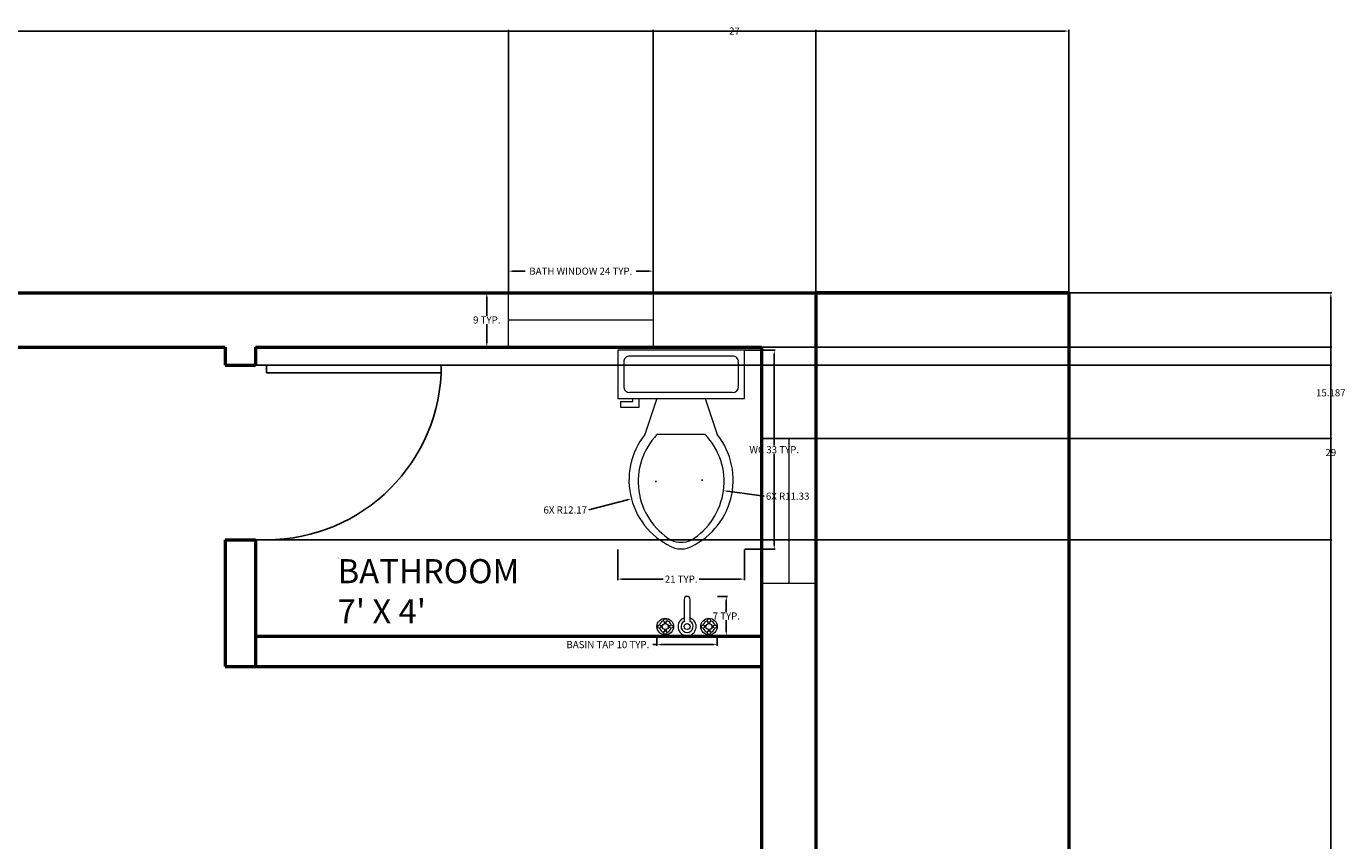
# Model space of a CAD drawing. Units: inches. Extents: x 3506 to 3958, y 1553 to 2506.
# Tile 16 of 16: x 3739 to 3958, y 2370 to 2506. Entities that reach past the tile are written whole.
import ezdxf

# ---------------------------------------------------------------- set-up
doc = ezdxf.new("R2010")
doc.units = ezdxf.units.IN
doc.header["$MEASUREMENT"] = 0
for name, color, linetype, lineweight in [('A-ANNO-DIMS', 2, 'Continuous', 18), ('A-AREA-IDEN', 7, 'Continuous', 18), ('A-WALL', 7, 'Continuous', 50), ('bathroom', 90, 'Continuous', 18), ('doors', 40, 'Continuous', 25), ('window', 30, 'Continuous', 20)]:
    doc.layers.add(name, color=color, linetype=linetype, lineweight=lineweight)
doc.layers.add('A-WALL-PATT', color=251, linetype='Continuous', lineweight=13, true_color=0x636466)
doc.styles.get("Standard").update_dxf_attribs({"font": 'arial.ttf'})
doc.dimstyles.get("Standard").update_dxf_attribs({"dimtxt": 1.18, "dimasz": 0.68, "dimexe": 0.18, "dimexo": 0.0625, "dimgap": 0.09, "dimtad": 0, "dimtih": 1, "dimtoh": 1, "dimdec": 1, "dimzin": 0, "dimdsep": 46, "dimlunit": 3, "dimtxsty": 'Standard', "dimcen": 0.09, "dimadec": 0, "dimazin": 0, "dimtfac": 1, "dimtdec": 1, "dimtofl": 0, "dimtmove": 0, "dimatfit": 3, "dimfxl": 1, "dimtolj": 1, "dimtzin": 0, "dimarcsym": 0})

# ---------------------------------------------------------------- blocks, each defined once
blk = doc.blocks.new('*U10')
for p, q in [((0, 0), (0, -6)), ((40, 0), (40, -6))]:
    blk.add_line(p, q)
blk.add_lwpolyline([(0, 0), (0, 40), (1.75, 40), (1.75, 0)], close=True)
blk.add_arc((0, 0), 40, 0, 90)
blk = doc.blocks.new('Toilet - top')
for p, q in [((9.5, -6), (9.5, -2)), ((-10, -8.5), (-8, -8.5)), ((-10, -9.5), (-10, -8.5)), ((-8, -8.5), (-8, -8)), ((-7, -8), (-7, -9.5)), ((-4, -8), (-6, -14)), ((4, -8), (6, -14)), ((-7, -9.5), (-10, -9.5)), ((4, -14), (-4, -14))]:
    blk.add_line(p, q)
blk.add_lwpolyline([(10.5, -8), (10.5, 0), (-10.5, 0), (-10.5, -8)], close=True)
for points in [[(-9.5, -2), (-9.5, -6)], [(8.5, -1), (-8.5, -1)], [(-8.5, -7), (8.5, -7)]]:
    blk.add_lwpolyline(points)
for centre, radius, start, end in [((-8.62, -1.88), 0.884, 81.8699, 188.1301), ((8.62, -1.88), 0.884, 351.8699, 98.1301), ((-8.62, -6.12), 0.884, 171.8699, 278.1301), ((8.62, -6.12), 0.884, 261.8699, 8.1301), ((3.52, -21.58), 12.17, 141.4691, 247.9714), ((4.2, -21.82), 11.33, 136.3677, 238.9468), ((-3.52, -21.58), 12.17, 292.0284, 38.5307), ((-4.2, -21.82), 11.33, 301.053, 43.6321), ((0, -27.88), 4, 245.7318, 294.2682), ((0, -29), 4, 254.8605, 285.1395)]:
    blk.add_arc(centre, radius, start, end)
blk = doc.blocks.new('Faucet - Bathroom top')
for p, q in [((-4.107, 0.125), (-4.375, 0.125)), ((-3.75, 0.4788), (-3.75, 0.75)), ((-3.5, 0.482), (-3.5, 0.75)), ((-3.1461, 0.125), (-2.875, 0.125)), ((3.143, 0.125), (2.875, 0.125)), ((3.5, 0.4788), (3.5, 0.75)), ((3.75, 0.482), (3.75, 0.75)), ((4.1039, 0.125), (4.375, 0.125)), ((-4.1039, -0.125), (-4.375, -0.125)), ((-3.75, -0.4821), (-3.75, -0.75)), ((-3.5, -0.4789), (-3.5, -0.75)), ((-3.143, -0.125), (-2.875, -0.125)), ((-0.5, -0.8639), (-0.5, -4.5)), ((0.5, -4.5), (0.5, -0.8631)), ((3.1461, -0.125), (2.875, -0.125)), ((3.5, -0.4821), (3.5, -0.75)), ((3.75, -0.4789), (3.75, -0.75)), ((4.107, -0.125), (4.375, -0.125))]:
    blk.add_line(p, q)
for centre, radius in [((-3.625, 0), 1.375), ((-4.625, 0), 0.2795), ((-3.625, 0), 0.5), ((-3.625, 1), 0.2795), ((-2.625, 0), 0.2795), ((0, 0), 0.5), ((3.625, 0), 1.375), ((2.625, 0), 0.2795), ((3.625, 0), 0.5), ((3.625, 1), 0.2795), ((4.625, 0), 0.2795), ((-3.625, -1), 0.2795), ((3.625, -1), 0.2795)]:
    blk.add_circle(centre, radius)
for centre, radius, start, end in [((-3.625, 0), 1, 105.2407, 164.2093), ((-3.625, 0), 1, 16.44125, 74.07887), ((0, 0), 1.5, 289.6514, 250.3603), ((0, 0), 1, 300.3431, 239.7554), ((3.625, 0), 1, 106.12, 164.0884), ((3.625, 0), 1, 16.23422, 73.90469), ((-3.625, 0), 1, 196.2342, 253.9047), ((-3.625, 0), 1, 286.12, 344.0884), ((3.625, 0), 1, 196.4413, 254.0789), ((3.625, 0), 1, 285.2407, 344.2093), ((0, -4.5), 0.5, 180, 0)]:
    blk.add_arc(centre, radius, start, end)
blk = doc.blocks.new('WIN-24IN-9IN-WALL')
for p, q in [((0, 0), (0, 9)), ((0, 9), (24, 9)), ((24, 9), (24, 0)), ((0, 0), (0, 4.5)), ((0, 4.5), (24, 4.5)), ((24, 0), (0, 0))]:
    blk.add_line(p, q)
blk = doc.blocks.new('*D26')
at = {"layer": 'A-ANNO-DIMS', "color": 0, "lineweight": -2, "transparency": 16777216}
for p, q in [((3857.94, 2451.88), (3863.01, 2451.88)), ((3862.83, 2451.2), (3862.83, 2436.05)), ((3862.83, 2419.51), (3862.83, 2434.65)), ((3857.94, 2418.83), (3863.01, 2418.83))]:
    blk.add_line(p, q, dxfattribs=at)
at = {"layer": 'A-ANNO-DIMS', "color": 0, "transparency": 16777216}
for points in [[(3862.72, 2451.2), (3862.95, 2451.2), (3862.83, 2451.88)], [(3862.72, 2419.51), (3862.95, 2419.51), (3862.83, 2418.83)]]:
    blk.add_solid(points, dxfattribs=at)
at = {"layer": 'Defpoints', "color": 0, "transparency": 16777216}
for p in [(3857.88, 2451.88), (3862.83, 2451.88), (3857.88, 2418.83)]:
    blk.add_point(p, dxfattribs=at)
at = {"layer": 'A-ANNO-DIMS', "color": 0, "transparency": 16777216, "insert": (3862.83, 2435.35), "char_height": 1.18, "attachment_point": 5}
blk.add_mtext('\\A1;WC 33 TYP.', dxfattribs=at)
blk = doc.blocks.new('*D27')
at = {"layer": 'A-ANNO-DIMS', "color": 0, "lineweight": -2, "transparency": 16777216}
for p, q in [((3836.88, 2418.77), (3836.88, 2413.69)), ((3857.88, 2418.77), (3857.88, 2413.69)), ((3837.55, 2413.87), (3844.4, 2413.87)), ((3857.2, 2413.87), (3850.35, 2413.87))]:
    blk.add_line(p, q, dxfattribs=at)
at = {"layer": 'A-ANNO-DIMS', "color": 0, "transparency": 16777216}
for points in [[(3837.55, 2413.99), (3837.55, 2413.76), (3836.88, 2413.87)], [(3857.2, 2413.99), (3857.2, 2413.76), (3857.88, 2413.87)]]:
    blk.add_solid(points, dxfattribs=at)
at = {"layer": 'Defpoints', "color": 0, "transparency": 16777216}
for p in [(3836.88, 2418.83), (3857.88, 2418.83), (3857.88, 2413.87)]:
    blk.add_point(p, dxfattribs=at)
at = {"layer": 'A-ANNO-DIMS', "color": 0, "transparency": 16777216, "insert": (3847.38, 2413.87), "char_height": 1.18, "attachment_point": 5}
blk.add_mtext('\\A1;21 TYP.', dxfattribs=at)
blk = doc.blocks.new('*D28')
at = {"layer": 'A-ANNO-DIMS', "color": 0, "lineweight": -2, "transparency": 16777216}
for p, q in [((3843.37, 2404.44), (3843.37, 2402.82)), ((3853.37, 2404.44), (3853.37, 2402.82)), ((3843.37, 2403), (3842.69, 2403)), ((3852.69, 2403), (3844.05, 2403))]:
    blk.add_line(p, q, dxfattribs=at)
at = {"layer": 'A-ANNO-DIMS', "color": 0, "transparency": 16777216}
for points in [[(3844.05, 2403.11), (3844.05, 2402.89), (3843.37, 2403)], [(3852.69, 2403.11), (3852.69, 2402.89), (3853.37, 2403)]]:
    blk.add_solid(points, dxfattribs=at)
at = {"layer": 'Defpoints', "color": 0, "transparency": 16777216}
for p in [(3843.37, 2404.5), (3853.37, 2404.5), (3843.37, 2403)]:
    blk.add_point(p, dxfattribs=at)
at = {"layer": 'A-ANNO-DIMS', "color": 0, "transparency": 16777216, "insert": (3835.22, 2403), "char_height": 1.18, "attachment_point": 5}
blk.add_mtext('\\A1;BASIN TAP 10 TYP.', dxfattribs=at)
blk = doc.blocks.new('*D29')
at = {"layer": 'A-ANNO-DIMS', "color": 0, "lineweight": -2, "transparency": 16777216}
for p, q in [((3853.44, 2411), (3855.06, 2411)), ((3854.88, 2410.32), (3854.88, 2408.43)), ((3854.88, 2405.18), (3854.88, 2407.07)), ((3853.44, 2404.5), (3855.06, 2404.5))]:
    blk.add_line(p, q, dxfattribs=at)
at = {"layer": 'A-ANNO-DIMS', "color": 0, "transparency": 16777216}
for points in [[(3854.76, 2410.32), (3854.99, 2410.32), (3854.88, 2411)], [(3854.76, 2405.18), (3854.99, 2405.18), (3854.88, 2404.5)]]:
    blk.add_solid(points, dxfattribs=at)
at = {"layer": 'Defpoints', "color": 0, "transparency": 16777216}
for p in [(3853.38, 2411), (3853.38, 2404.5), (3854.88, 2404.5)]:
    blk.add_point(p, dxfattribs=at)
at = {"layer": 'A-ANNO-DIMS', "color": 0, "transparency": 16777216, "insert": (3854.88, 2407.75), "char_height": 1.18, "attachment_point": 5}
blk.add_mtext('\\A1;7 TYP.', dxfattribs=at)
blk = doc.blocks.new('*D30')
at = {"layer": 'A-ANNO-DIMS', "color": 0, "lineweight": -2, "transparency": 16777216}
for p, q in [((3818.73, 2461.46), (3818.73, 2465.17)), ((3819.41, 2464.99), (3821.52, 2464.99)), ((3842.05, 2464.99), (3839.94, 2464.99)), ((3842.73, 2461.46), (3842.73, 2465.17))]:
    blk.add_line(p, q, dxfattribs=at)
at = {"layer": 'A-ANNO-DIMS', "color": 0, "transparency": 16777216}
for points in [[(3819.41, 2465.11), (3819.41, 2464.88), (3818.73, 2464.99)], [(3842.05, 2465.11), (3842.05, 2464.88), (3842.73, 2464.99)]]:
    blk.add_solid(points, dxfattribs=at)
at = {"layer": 'Defpoints', "color": 0, "transparency": 16777216}
for p in [(3842.73, 2464.99), (3818.73, 2461.39), (3842.73, 2461.39)]:
    blk.add_point(p, dxfattribs=at)
at = {"layer": 'A-ANNO-DIMS', "color": 0, "transparency": 16777216, "insert": (3830.73, 2464.99), "char_height": 1.18, "attachment_point": 5}
blk.add_mtext('\\A1;BATH WINDOW 24 TYP.', dxfattribs=at)
blk = doc.blocks.new('*D31')
at = {"layer": 'A-ANNO-DIMS', "color": 0, "lineweight": -2, "transparency": 16777216}
for p, q in [((3818.67, 2461.39), (3814.95, 2461.39)), ((3815.13, 2460.71), (3815.13, 2457.59)), ((3815.13, 2453.07), (3815.13, 2456.2)), ((3818.67, 2452.39), (3814.95, 2452.39))]:
    blk.add_line(p, q, dxfattribs=at)
at = {"layer": 'A-ANNO-DIMS', "color": 0, "transparency": 16777216}
for points in [[(3815.02, 2460.71), (3815.24, 2460.71), (3815.13, 2461.39)], [(3815.02, 2453.07), (3815.24, 2453.07), (3815.13, 2452.39)]]:
    blk.add_solid(points, dxfattribs=at)
at = {"layer": 'Defpoints', "color": 0, "transparency": 16777216}
for p in [(3815.13, 2461.39), (3818.73, 2461.39), (3818.73, 2452.39)]:
    blk.add_point(p, dxfattribs=at)
at = {"layer": 'A-ANNO-DIMS', "color": 0, "transparency": 16777216, "insert": (3815.13, 2456.89), "char_height": 1.18, "attachment_point": 5}
blk.add_mtext('\\A1;9 TYP.', dxfattribs=at)
blk = doc.blocks.new('*D38')
at = {"layer": 'A-ANNO-DIMS', "color": 0, "lineweight": -2, "transparency": 16777216}
for p, q in [((3551.73, 2461.46), (3551.73, 2505.02)), ((3552.41, 2504.84), (3730.34, 2504.84)), ((3911.05, 2504.84), (3733.12, 2504.84)), ((3911.73, 2461.46), (3911.73, 2505.02))]:
    blk.add_line(p, q, dxfattribs=at)
at = {"layer": 'A-ANNO-DIMS', "color": 0, "transparency": 16777216}
for points in [[(3552.41, 2504.96), (3552.41, 2504.73), (3551.73, 2504.84)], [(3911.05, 2504.96), (3911.05, 2504.73), (3911.73, 2504.84)]]:
    blk.add_solid(points, dxfattribs=at)
at = {"layer": 'Defpoints', "color": 0, "transparency": 16777216}
for p in [(3911.73, 2504.84), (3551.73, 2461.39), (3911.73, 2461.39)]:
    blk.add_point(p, dxfattribs=at)
at = {"layer": 'A-ANNO-DIMS', "color": 0, "transparency": 16777216, "insert": (3731.73, 2504.84), "char_height": 1.18, "attachment_point": 5}
blk.add_mtext('\\A1;360', dxfattribs=at)
blk = doc.blocks.new('*D39')
at = {"layer": 'A-ANNO-DIMS', "color": 0, "lineweight": -2, "transparency": 16777216}
for p, q in [((3911.79, 2461.39), (3955.36, 2461.39)), ((3955.18, 2460.71), (3955.18, 2030.09)), ((3955.18, 1598.07), (3955.18, 2028.7)), ((3911.79, 1597.39), (3955.36, 1597.39))]:
    blk.add_line(p, q, dxfattribs=at)
at = {"layer": 'A-ANNO-DIMS', "color": 0, "transparency": 16777216}
for points in [[(3955.07, 2460.71), (3955.29, 2460.71), (3955.18, 2461.39)], [(3955.07, 1598.07), (3955.29, 1598.07), (3955.18, 1597.39)]]:
    blk.add_solid(points, dxfattribs=at)
at = {"layer": 'Defpoints', "color": 0, "transparency": 16777216}
for p in [(3911.73, 2461.39), (3955.18, 2461.39), (3911.73, 1597.39)]:
    blk.add_point(p, dxfattribs=at)
at = {"layer": 'A-ANNO-DIMS', "color": 0, "transparency": 16777216, "insert": (3955.18, 2029.39), "char_height": 1.18, "attachment_point": 5}
blk.add_mtext('\\A1;864', dxfattribs=at)
blk = doc.blocks.new('*D44')
at = {"layer": 'A-ANNO-DIMS', "color": 0, "lineweight": -2, "transparency": 16777216}
for p, q in [((3911.67, 2461.39), (3508.1, 2461.39)), ((3508.28, 2460.71), (3508.28, 2344.59)), ((3508.28, 2227.07), (3508.28, 2343.2)), ((3560.67, 2226.39), (3508.1, 2226.39))]:
    blk.add_line(p, q, dxfattribs=at)
at = {"layer": 'A-ANNO-DIMS', "color": 0, "transparency": 16777216}
for points in [[(3508.17, 2460.71), (3508.39, 2460.71), (3508.28, 2461.39)], [(3508.17, 2227.07), (3508.39, 2227.07), (3508.28, 2226.39)]]:
    blk.add_solid(points, dxfattribs=at)
at = {"layer": 'Defpoints', "color": 0, "transparency": 16777216}
for p in [(3508.28, 2461.39), (3911.73, 2461.39), (3560.73, 2226.39)]:
    blk.add_point(p, dxfattribs=at)
at = {"layer": 'A-ANNO-DIMS', "color": 0, "transparency": 16777216, "insert": (3508.28, 2343.89), "char_height": 1.18, "attachment_point": 5}
blk.add_mtext('\\A1;235', dxfattribs=at)
blk = doc.blocks.new('*D46')
at = {"layer": 'A-ANNO-DIMS', "color": 0, "lineweight": -2, "transparency": 16777216}
for p, q in [((3643.67, 2461.46), (3643.67, 2505.02)), ((3644.35, 2504.84), (3728.72, 2504.84)), ((3818.05, 2504.84), (3733.68, 2504.84)), ((3818.73, 2461.46), (3818.73, 2505.02))]:
    blk.add_line(p, q, dxfattribs=at)
at = {"layer": 'A-ANNO-DIMS', "color": 0, "transparency": 16777216}
for points in [[(3644.35, 2504.96), (3644.35, 2504.73), (3643.67, 2504.84)], [(3818.05, 2504.96), (3818.05, 2504.73), (3818.73, 2504.84)]]:
    blk.add_solid(points, dxfattribs=at)
at = {"layer": 'Defpoints', "color": 0, "transparency": 16777216}
for p in [(3818.73, 2504.84), (3643.67, 2461.39), (3818.73, 2461.39)]:
    blk.add_point(p, dxfattribs=at)
at = {"layer": 'A-ANNO-DIMS', "color": 0, "transparency": 16777216, "insert": (3731.2, 2504.84), "char_height": 1.18, "attachment_point": 5}
blk.add_mtext('\\A1;175.06', dxfattribs=at)
blk = doc.blocks.new('*D47')
at = {"layer": 'A-ANNO-DIMS', "color": 0, "lineweight": -2, "transparency": 16777216}
for p, q in [((3842.73, 2461.46), (3842.73, 2505.02)), ((3843.41, 2504.84), (3855.28, 2504.84)), ((3869.05, 2504.84), (3857.18, 2504.84)), ((3869.73, 2461.46), (3869.73, 2505.02))]:
    blk.add_line(p, q, dxfattribs=at)
at = {"layer": 'A-ANNO-DIMS', "color": 0, "transparency": 16777216}
for points in [[(3843.41, 2504.96), (3843.41, 2504.73), (3842.73, 2504.84)], [(3869.05, 2504.96), (3869.05, 2504.73), (3869.73, 2504.84)]]:
    blk.add_solid(points, dxfattribs=at)
at = {"layer": 'Defpoints', "color": 0, "transparency": 16777216}
for p in [(3869.73, 2504.84), (3842.73, 2461.39), (3869.73, 2461.39)]:
    blk.add_point(p, dxfattribs=at)
at = {"layer": 'A-ANNO-DIMS', "color": 0, "transparency": 16777216, "insert": (3856.23, 2504.84), "char_height": 1.18, "attachment_point": 5}
blk.add_mtext('\\A1;27', dxfattribs=at)
blk = doc.blocks.new('*D53')
at = {"layer": 'A-ANNO-DIMS', "color": 0, "lineweight": -2, "transparency": 16777216}
for p, q in [((3860.79, 2452.39), (3955.36, 2452.39)), ((3955.18, 2451.71), (3955.18, 2445.49)), ((3955.18, 2437.89), (3955.18, 2444.11)), ((3860.79, 2437.21), (3955.36, 2437.21))]:
    blk.add_line(p, q, dxfattribs=at)
at = {"layer": 'A-ANNO-DIMS', "color": 0, "transparency": 16777216}
for points in [[(3955.07, 2451.71), (3955.29, 2451.71), (3955.18, 2452.39)], [(3955.07, 2437.89), (3955.29, 2437.89), (3955.18, 2437.21)]]:
    blk.add_solid(points, dxfattribs=at)
at = {"layer": 'Defpoints', "color": 0, "transparency": 16777216}
for p in [(3860.73, 2452.39), (3860.73, 2437.21), (3955.18, 2437.21)]:
    blk.add_point(p, dxfattribs=at)
at = {"layer": 'A-ANNO-DIMS', "color": 0, "transparency": 16777216, "insert": (3955.18, 2444.8), "char_height": 1.18, "attachment_point": 5}
blk.add_mtext('\\A1;15.187', dxfattribs=at)
blk = doc.blocks.new('*D57')
at = {"layer": 'A-ANNO-DIMS', "color": 0, "lineweight": -2, "transparency": 16777216}
for p, q in [((3776.79, 2449.39), (3955.36, 2449.39)), ((3955.18, 2448.71), (3955.18, 2435.59)), ((3955.18, 2421.07), (3955.18, 2434.2)), ((3776.79, 2420.39), (3955.36, 2420.39))]:
    blk.add_line(p, q, dxfattribs=at)
at = {"layer": 'A-ANNO-DIMS', "color": 0, "transparency": 16777216}
for points in [[(3955.07, 2448.71), (3955.29, 2448.71), (3955.18, 2449.39)], [(3955.07, 2421.07), (3955.29, 2421.07), (3955.18, 2420.39)]]:
    blk.add_solid(points, dxfattribs=at)
at = {"layer": 'Defpoints', "color": 0, "transparency": 16777216}
for p in [(3776.73, 2449.39), (3776.73, 2420.39), (3955.18, 2420.39)]:
    blk.add_point(p, dxfattribs=at)
at = {"layer": 'A-ANNO-DIMS', "color": 0, "transparency": 16777216, "insert": (3955.18, 2434.89), "char_height": 1.18, "attachment_point": 5}
blk.add_mtext('\\A1;29', dxfattribs=at)
blk = doc.blocks.new('*D73')
at = {"layer": 'A-ANNO-DIMS', "color": 0, "lineweight": -2, "transparency": 16777216}
for p, q in [((3850.8, 2430.29), (3850.98, 2430.29)), ((3850.89, 2430.2), (3850.89, 2430.38)), ((3832.06, 2425.35), (3838.47, 2427.03))]:
    blk.add_line(p, q, dxfattribs=at)
at = {"layer": 'A-ANNO-DIMS', "color": 0, "transparency": 16777216}
blk.add_solid([(3838.44, 2427.14), (3838.5, 2426.92), (3839.13, 2427.2)], dxfattribs=at)
at = {"layer": 'Defpoints', "color": 0, "transparency": 16777216}
for p in [(3850.89, 2430.29), (3839.13, 2427.2)]:
    blk.add_point(p, dxfattribs=at)
at = {"layer": 'A-ANNO-DIMS', "color": 0, "transparency": 16777216, "insert": (3828.15, 2425.35), "char_height": 1.18, "attachment_point": 5}
blk.add_mtext('\\A1;6X R12.17', dxfattribs=at)
blk = doc.blocks.new('*D74')
at = {"layer": 'A-ANNO-DIMS', "color": 0, "lineweight": -2, "transparency": 16777216}
for p, q in [((3843.09, 2430.06), (3843.27, 2430.06)), ((3843.18, 2429.97), (3843.18, 2430.15)), ((3861.14, 2427.64), (3855.08, 2428.46))]:
    blk.add_line(p, q, dxfattribs=at)
at = {"layer": 'A-ANNO-DIMS', "color": 0, "transparency": 16777216}
blk.add_solid([(3855.09, 2428.57), (3855.06, 2428.35), (3854.4, 2428.55)], dxfattribs=at)
at = {"layer": 'Defpoints', "color": 0, "transparency": 16777216}
for p in [(3843.18, 2430.06), (3854.4, 2428.55)]:
    blk.add_point(p, dxfattribs=at)
at = {"layer": 'A-ANNO-DIMS', "color": 0, "transparency": 16777216, "insert": (3865.06, 2427.64), "char_height": 1.18, "attachment_point": 5}
blk.add_mtext('\\A1;6X R11.33', dxfattribs=at)

msp = doc.modelspace()

# ---------------------------------------------------------------- hatches: boundary and pattern name
at = {"layer": 'A-WALL-PATT'}
h = msp.add_hatch(dxfattribs=at)
h.set_pattern_fill('ANSI31', color=256)
h.paths.add_polyline_path([(3911.7302, 2461.3942), (3551.7302, 2461.3942), (3551.7302, 2152.516), (3560.7302, 2152.516), (3560.7302, 2116.516), (3551.7302, 2116.516), (3551.7302, 1920.5711), (3556.2302, 1920.5711), (3560.7302, 1920.5711), (3560.7302, 2000.3942), (3692.7302, 2000.3942), (3692.7302, 1997.3942), (3697.7302, 1997.3942), (3697.7302, 2000.3942), (3771.7302, 2000.3942), (3771.7302, 1997.3942), (3776.7302, 1997.3942), (3776.7302, 1997.7206), (3778.5802, 1997.7206), (3807.5802, 1997.7206), (3807.5802, 1996.4519), (3778.5802, 1996.4519), (3778.5802, 1997.7206), (3776.7302, 1997.7206), (3776.7302, 1997.3942), (3771.7302, 1997.3942), (3771.7302, 2000.3942), (3697.7302, 2000.3942), (3697.7302, 1997.3942), (3692.7302, 1997.3942), (3689.8302, 1997.3942), (3689.8302, 1995.8192), (3653.8302, 1995.8192), (3653.8302, 1997.3942), (3689.8302, 1997.3942), (3692.7302, 1997.3942), (3692.7302, 2000.3942), (3560.7302, 2000.3942), (3560.7302, 1920.5711), (3551.7302, 1920.5711), (3551.7302, 1884.5711), (3551.7302, 1597.3942), (3911.7302, 1597.3942)], flags=17)
h.paths.add_polyline_path([(3596.7302, 2005.3942), (3596.7302, 2057.3035, -0.38730371), (3569.1778, 2085), (3569.15, 2085), (3569.15, 2086.2688), (3598.15, 2086.2688), (3598.15, 2085), (3569.1778, 2085, 0.38730371), (3596.7302, 2057.3035), (3596.7302, 2057.3942), (3601.7302, 2057.3942), (3601.7302, 2055.3942), (3630.7302, 2055.3942), (3630.7302, 2034.3942), (3694.7302, 2034.3942), (3694.7302, 2053.3942), (3699.7302, 2053.3942), (3699.7302, 2005.3942), (3860.7302, 2005.3942), (3860.7302, 2173.3942), (3771.7302, 2173.3942), (3771.7302, 2194.3942), (3776.7302, 2194.3942), (3776.7302, 2178.3942), (3860.7302, 2178.3942), (3860.7302, 2231.3942), (3601.7302, 2231.3942), (3601.7302, 2241.426), (3596.7302, 2241.426), (3596.7302, 2231.3942), (3560.7302, 2231.3942), (3560.7302, 2315.3942), (3596.7302, 2315.3942), (3596.7302, 2312.3942), (3601.7302, 2312.3942), (3601.7302, 2315.3942), (3697.7302, 2315.3942), (3697.7302, 2413.3942), (3692.7302, 2413.3942), (3692.7302, 2320.3942), (3560.7302, 2320.3942), (3560.7302, 2452.3942), (3692.7302, 2452.3942), (3692.7302, 2449.3942), (3697.7302, 2449.3942), (3697.7302, 2452.3942), (3771.7302, 2452.3942), (3771.7302, 2449.3942), (3776.7302, 2449.3942), (3776.7302, 2452.3942), (3860.7302, 2452.3942), (3860.7302, 2437.2075), (3865.2302, 2437.2075), (3865.2302, 2413.2075), (3860.7302, 2413.2075), (3860.7302, 2367.6976), (3865.2302, 2367.6976), (3869.7302, 2367.6976), (3869.7302, 2319.6976), (3860.7302, 2319.6976), (3860.7302, 2211.6248), (3869.7302, 2211.6248), (3869.7302, 2187.6248), (3860.7302, 2187.6248), (3860.7302, 2138.4346), (3865.2302, 2138.4346), (3869.7302, 2138.4346), (3869.7302, 2090.4346), (3860.7302, 2090.4346), (3860.7302, 1985.8449), (3869.7302, 1985.8449), (3869.7302, 1961.8449), (3860.7302, 1961.8449), (3860.7302, 1897.0756), (3865.2302, 1897.0756), (3869.7302, 1897.0756), (3869.7302, 1849.0756), (3860.7302, 1849.0756), (3860.7302, 1847.8112), (3860.7302, 1779.3942), (3596.7302, 1779.3942), (3596.7302, 1831.3942), (3601.7302, 1831.3942), (3601.7302, 1828.3942), (3630.7302, 1828.3942), (3630.7302, 1808.3942), (3691.7302, 1808.3942), (3691.7302, 1815.3942), (3696.7302, 1815.3942), (3696.7302, 1779.3942), (3860.7302, 1779.3942), (3860.7302, 1947.3942), (3771.7302, 1947.3942), (3771.7302, 1968.3942), (3776.7302, 1968.3942), (3776.7302, 1952.3942), (3860.7302, 1952.3942), (3860.7302, 2005.3942)], flags=0)
h.paths.add_polyline_path([(3596.7302, 2038.8546), (3601.7302, 2038.8546), (3601.7302, 2014.8546), (3596.7302, 2014.8546)], flags=0)
h.paths.add_polyline_path([(3564.1688, 2107), (3564.1688, 2167), (3644.1688, 2167), (3644.1688, 2107)], flags=0)
h.paths.add_polyline_path([(3607.0972, 2052.0208), (3620.8472, 2052.0208, -0.41421356), (3621.9931, 2050.875), (3621.9931, 2025.6667, -0.41421356), (3620.8472, 2024.5208), (3607.0972, 2024.5208, -0.41421356), (3605.9514, 2025.6667), (3605.9514, 2050.875, -0.41421356)], flags=0)
h.paths.add_polyline_path([(3578.5688, 2115), (3565.3688, 2115), (3565.3688, 2135.8), (3578.5688, 2135.8), (3578.5688, 2138.2), (3565.3688, 2138.2), (3565.3688, 2159), (3580.5688, 2159), (3580.5688, 2153.8), (3593.7688, 2167), (3593.7688, 2151.8), (3578.5688, 2151.8)], flags=0)
h.paths.add_polyline_path([(3610.9167, 2050.875), (3620.0833, 2050.875, -0.41421356), (3620.8472, 2050.1111), (3620.8472, 2039.6076, -0.41421356), (3620.0833, 2038.8438), (3610.9167, 2038.8438, -0.41421356), (3610.1528, 2039.6076), (3610.1528, 2050.1111, -0.41421356)], flags=0)
h.paths.add_polyline_path([(3610.9167, 2037.6979), (3620.0833, 2037.6979, -0.41421356), (3620.8472, 2036.934), (3620.8472, 2026.4306, -0.41421356), (3620.0833, 2025.6667), (3610.9167, 2025.6667, -0.41421356), (3610.1528, 2026.4306), (3610.1528, 2036.934, -0.41421356)], flags=0)
h.paths.add_polyline_path([(3616.2639, 2044.7639, -1), (3614.7361, 2044.7639, -1)], flags=0)
h.paths.add_polyline_path([(3615.8819, 2044.7639, -1), (3615.1181, 2044.7639, -1)], flags=0)
h.paths.add_polyline_path([(3616.2639, 2031.7778, -1), (3614.7361, 2031.7778, -1)], flags=0)
h.paths.add_polyline_path([(3615.8819, 2031.7778, -1), (3615.1181, 2031.7778, -1)], flags=0)
h.paths.add_polyline_path([(3609.7539, 2021.7868), (3626.9586, 2021.7868), (3626.9586, 2008.8833), (3609.7539, 2008.8833)], flags=0)
h.paths.add_polyline_path([(3610.4708, 2021.07), (3621.2237, 2021.07), (3621.2237, 2009.6002), (3610.4708, 2009.6002)], flags=0)
h.paths.add_polyline_path([(3611.5461, 2019.9947), (3620.1484, 2019.9947), (3620.1484, 2010.6755), (3611.5461, 2010.6755)], flags=0)
h.paths.add_polyline_path([(3621.9405, 2021.07), (3626.2417, 2021.07), (3626.2417, 2009.6002), (3621.9405, 2009.6002)], flags=0)
h.paths.add_polyline_path([(3622.6574, 2020.3531), (3625.5248, 2020.3531), (3625.5248, 2017.4857), (3622.6574, 2017.4857)], flags=0)
h.paths.add_polyline_path([(3622.6574, 2016.7688), (3625.5248, 2016.7688), (3625.5248, 2010.317), (3622.6574, 2010.317)], flags=0)
h.paths.add_polyline_path([(3624.808, 2016.0519), (3624.808, 2013.9013), (3624.0911, 2013.9013), (3624.0911, 2013.1845), (3623.3743, 2013.1845), (3623.3743, 2013.9013), (3623.3743, 2016.0519)], flags=0)
h.paths.add_polyline_path([(3623.0158, 2012.8261), (3625.1664, 2012.8261), (3625.1664, 2012.1092), (3623.0158, 2012.1092)], flags=0)
h.paths.add_polyline_path([(3623.0158, 2011.7508), (3625.1664, 2011.7508), (3625.1664, 2011.0339), (3623.0158, 2011.0339)], flags=0)
h.paths.add_polyline_path([(3650.0591, 2031.8202), (3674.0368, 2031.8202), (3674.0368, 2012.638), (3669.2413, 2012.638), (3669.2413, 2011.8388), (3672.4383, 2011.8388), (3672.4383, 2011.0395), (3651.6576, 2011.0395), (3651.6576, 2011.8388), (3654.8546, 2011.8388), (3654.8546, 2012.638), (3650.0591, 2012.638)], flags=0)
h.paths.add_polyline_path([(3658.0517, 2024.6269, -1), (3651.6576, 2024.6269, -1)], flags=0)
h.paths.add_polyline_path([(3657.2524, 2024.6269, -1), (3652.4569, 2024.6269, -1)], flags=0)
h.paths.add_polyline_path([(3656.4532, 2024.6269, -1), (3653.2561, 2024.6269, -1)], flags=0)
h.paths.add_polyline_path([(3655.6539, 2024.6269, -1), (3654.0554, 2024.6269, -1)], flags=0)
h.paths.add_polyline_path([(3657.2524, 2017.4336, -1), (3652.4569, 2017.4336, -1)], flags=0)
h.paths.add_polyline_path([(3656.4532, 2017.4336, -1), (3653.2561, 2017.4336, -1)], flags=0)
h.paths.add_polyline_path([(3655.6539, 2017.4336, -1), (3654.0554, 2017.4336, -1)], flags=0)
h.paths.add_polyline_path([(3659.6502, 2027.8239), (3664.4457, 2027.8239), (3664.4457, 2015.0358), (3659.6502, 2015.0358)], flags=0)
h.paths.add_polyline_path([(3663.6465, 2027.0247), (3663.6465, 2015.8351), (3660.4494, 2015.8351), (3660.4494, 2027.0247)], flags=0)
h.paths.add_polyline_path([(3562.6688, 1945.5), (3642.6688, 1945.5), (3642.6688, 1885.5), (3562.6688, 1885.5)], flags=0)
h.paths.add_polyline_path([(3671.6391, 2024.6269, -1), (3666.8435, 2024.6269, -1)], flags=0)
h.paths.add_polyline_path([(3670.8398, 2024.6269, -1), (3667.6428, 2024.6269, -1)], flags=0)
h.paths.add_polyline_path([(3672.4383, 2017.4336, -1), (3666.0443, 2017.4336, -1)], flags=0)
h.paths.add_polyline_path([(3670.0405, 2024.6269, -1), (3668.442, 2024.6269, -1)], flags=0)
h.paths.add_polyline_path([(3671.6391, 2017.4336, -1), (3666.8435, 2017.4336, -1)], flags=0)
h.paths.add_polyline_path([(3670.8398, 2017.4336, -1), (3667.6428, 2017.4336, -1)], flags=0)
h.paths.add_polyline_path([(3592.2688, 1945.5), (3592.2688, 1930.3), (3577.0688, 1930.3), (3577.0688, 1893.5), (3563.8688, 1893.5), (3563.8688, 1914.3), (3577.0688, 1914.3), (3577.0688, 1916.7), (3563.8688, 1916.7), (3563.8688, 1937.5), (3579.0688, 1937.5), (3579.0688, 1932.3)], flags=0)
h.paths.add_polyline_path([(3670.0405, 2017.4336, -1), (3668.442, 2017.4336, -1)], flags=0)
h.paths.add_polyline_path([(3596.7302, 2283.3942), (3601.7302, 2283.3942), (3601.7302, 2265.426), (3599.2302, 2265.426), (3599.2302, 2241.426), (3596.7302, 2241.426), (3596.7302, 2265.426)], flags=0)
h.paths.add_polyline_path([(3596.7302, 1810.7006), (3601.7302, 1810.7006), (3601.7302, 1786.7006), (3596.7302, 1786.7006)], flags=0)
h.paths.add_polyline_path([(3560.7302, 1770.3942), (3738.7302, 1770.3942), (3738.7302, 1746.3942), (3738.7302, 1722.3942), (3748.7302, 1722.3942), (3748.7302, 1674.3942), (3560.7302, 1674.3942)], flags=0)
h.paths.add_polyline_path([(3728.7302, 1746.3942), (3728.7302, 1756.0642), (3738.7302, 1746.3942), (3728.7302, 1738.1582), (3728.7302, 1698.3942), (3591.2519, 1698.3942), (3591.2519, 1746.3942)], flags=0)
h.paths.add_polyline_path([(3771.7302, 2399.3942), (3771.7302, 2420.3942), (3776.7302, 2420.3942), (3776.7302, 2404.3942), (3776.7302, 2399.3942)], flags=0)
h.paths.add_polyline_path([(3911.7302, 2461.3942), (3551.7302, 2461.3942), (3551.7302, 2152.516), (3560.7302, 2152.516), (3560.7302, 2116.516), (3551.7302, 2116.516), (3551.7302, 1920.5711), (3560.7302, 1920.5711), (3560.7302, 2000.3942), (3692.7302, 2000.3942), (3692.7302, 1997.3942), (3697.7302, 1997.3942), (3697.7302, 2000.3942), (3771.7302, 2000.3942), (3771.7302, 1997.3942), (3776.7302, 1997.3942), (3776.7302, 1997.7206), (3778.5802, 1997.7206), (3807.5802, 1997.7206), (3807.5802, 1996.4519), (3778.5802, 1996.4519), (3778.5802, 1997.7206), (3776.7302, 1997.7206), (3776.7302, 1997.3942), (3771.7302, 1997.3942), (3771.7302, 2000.3942), (3697.7302, 2000.3942), (3697.7302, 1997.3942), (3692.7302, 1997.3942), (3689.8302, 1997.3942), (3689.8302, 1995.8192), (3653.8302, 1995.8192), (3653.8302, 1997.3942), (3689.8302, 1997.3942), (3692.7302, 1997.3942), (3692.7302, 2000.3942), (3560.7302, 2000.3942), (3560.7302, 1920.5711), (3551.7302, 1920.5711), (3551.7302, 1597.3942), (3911.7302, 1597.3942)], flags=17)

# ---------------------------------------------------------------- linework, layer by layer
at = {"layer": 'A-WALL'}
for p, q in [((3911.7302, 2461.3942), (3869.7302, 2461.3942)), ((3869.7302, 2461.3942), (3869.7302, 2297.8816)), ((3697.7302, 2452.3942), (3771.7302, 2452.3942)), ((3771.7302, 2452.3942), (3771.7302, 2449.3942)), ((3771.7302, 2452.3942), (3771.7302, 2449.3942)), ((3771.7302, 2452.3942), (3771.7302, 2449.3942)), ((3771.7302, 2452.3942), (3771.7302, 2449.3942)), ((3776.7302, 2452.3942), (3776.7302, 2449.3942)), ((3776.7302, 2452.3942), (3776.7302, 2449.3942)), ((3776.7302, 2452.3942), (3776.7302, 2449.3942)), ((3776.7302, 2452.3942), (3860.7302, 2452.3942)), ((3860.7302, 2452.3942), (3860.7302, 2297.8816)), ((3771.7302, 2449.3942), (3776.7302, 2449.3942)), ((3771.7302, 2420.3942), (3776.7302, 2420.3942)), ((3771.7302, 2420.3942), (3771.7302, 2399.3942)), ((3771.7302, 2420.3942), (3771.7302, 2399.3942)), ((3771.7302, 2420.3942), (3771.7302, 2399.3942)), ((3776.7302, 2420.3942), (3776.7302, 2399.3942)), ((3776.7302, 2420.3942), (3776.7302, 2404.3942)), ((3776.7302, 2420.3942), (3776.7302, 2399.3942)), ((3776.7302, 2404.3942), (3860.7302, 2404.3942)), ((3771.7302, 2399.3942), (3860.7302, 2399.3942))]:
    msp.add_line(p, q, dxfattribs=at)
msp.add_lwpolyline([(3551.7302, 2461.3942), (3911.7302, 2461.3942), (3911.7302, 1597.3942), (3551.7302, 1597.3942)], close=True, dxfattribs=at)
at = {"layer": 'window'}
for p, q in [((3869.7302, 2437.2075), (3860.7302, 2437.2075)), ((3860.7302, 2437.2075), (3860.7302, 2413.2075)), ((3865.2302, 2437.2075), (3865.2302, 2413.2075)), ((3860.7302, 2413.2075), (3869.7302, 2413.2075)), ((3860.7302, 2413.2075), (3865.2302, 2413.2075))]:
    msp.add_line(p, q, dxfattribs=at)

# ---------------------------------------------------------------- block references
at = {"layer": 'bathroom'}
msp.add_blockref('Toilet - top', (3847.375, 2451.875), dxfattribs=at)
at = {"layer": 'bathroom', "rotation": 180}
msp.add_blockref('Faucet - Bathroom top', (3848.375, 2406), dxfattribs=at)
at = {"layer": 'doors', "xscale": 0.725, "yscale": 0.725, "zscale": 0.725, "rotation": 270}
msp.add_blockref('*U10', (3778.5802, 2449.3942), dxfattribs=at)
at = {"layer": 'window'}
msp.add_blockref('WIN-24IN-9IN-WALL', (3818.73, 2452.394), dxfattribs=at)

# ---------------------------------------------------------------- texts
at = {"layer": 'A-AREA-IDEN', "insert": (3790.3788, 2417.5222), "char_height": 0.2, "attachment_point": 1}
msp.add_mtext_dynamic_manual_height_columns('4"\\P{\\H20x;BATHROOM\\P7\' X 4\'}', width=25.775469, gutter_width=1, heights=[0], dxfattribs=at)

# ---------------------------------------------------------------- dimensions: what is measured, and where the dimension line sits
at = {"layer": 'A-ANNO-DIMS'}
for base, p1, p2, override, picture, middle in [((3911.7302, 2504.8442), (3551.7302, 2461.3942), (3911.7302, 2461.3942), {"dimdec": 0, "dimlfac": 1, "dimrnd": 0, "dimzin": 0, "dimdsep": 46, "dimlunit": 2}, '*D38', (3731.7302, 2504.8442)), ((3818.7302, 2504.8442), (3643.667, 2461.3942), (3818.7302, 2461.3942), {"dimdec": 2, "dimlfac": 1, "dimrnd": 0, "dimzin": 0, "dimdsep": 46, "dimlunit": 2}, '*D46', (3731.1986, 2504.8442)), ((3869.7302, 2504.8442), (3842.7302, 2461.3942), (3869.7302, 2461.3942), {"dimdec": 0, "dimlfac": 1, "dimrnd": 0, "dimzin": 0, "dimdsep": 46, "dimlunit": 2}, '*D47', (3856.2302, 2504.8442))]:
    dim = msp.add_linear_dim(base=base, p1=p1, p2=p2, dimstyle='Standard', override=override, dxfattribs=at)
    dim.commit()
    dim.dimension.update_dxf_attribs({"geometry": picture, "text_midpoint": middle})
for base, p1, p2, text, picture, middle in [((3842.7302, 2464.9942), (3818.7302, 2461.3942), (3842.7302, 2461.3942), 'BATH WINDOW <> TYP.', '*D30', (3830.7302, 2464.9942)), ((3857.875, 2413.8718), (3836.875, 2418.8288), (3857.875, 2418.8288), '<> TYP.', '*D27', (3847.375, 2413.8718))]:
    dim = msp.add_linear_dim(base=base, p1=p1, p2=p2, text=text, dimstyle='Standard', override={"dimdec": 0, "dimlfac": 1, "dimrnd": 0, "dimzin": 0, "dimdsep": 46, "dimlunit": 2}, dxfattribs=at)
    dim.commit()
    dim.dimension.update_dxf_attribs({"geometry": picture, "text_midpoint": middle})
for base, p1, p2, override, picture, middle in [((3508.2802, 2461.3942), (3560.7302, 2226.3942), (3911.7302, 2461.3942), {"dimdec": 0, "dimlfac": 1, "dimrnd": 0, "dimzin": 0, "dimdsep": 46, "dimlunit": 2}, '*D44', (3508.2802, 2343.8942)), ((3955.1802, 2461.3942), (3911.7302, 1597.3942), (3911.7302, 2461.3942), {"dimdec": 0, "dimlfac": 1, "dimrnd": 0, "dimzin": 0, "dimdsep": 46, "dimlunit": 2}, '*D39', (3955.1802, 2029.3942)), ((3955.1802, 2437.2075), (3860.7302, 2452.3942), (3860.7302, 2437.2075), {"dimdec": 3, "dimlfac": 1, "dimrnd": 0, "dimzin": 0, "dimdsep": 46, "dimlunit": 2}, '*D53', (3955.1802, 2444.8008)), ((3955.1802, 2420.3942), (3776.7302, 2449.3942), (3776.7302, 2420.3942), {"dimdec": 0, "dimlfac": 1, "dimrnd": 0, "dimzin": 0, "dimdsep": 46, "dimlunit": 2}, '*D57', (3955.1802, 2434.8942))]:
    dim = msp.add_linear_dim(base=base, p1=p1, p2=p2, angle=90, dimstyle='Standard', override=override, dxfattribs=at)
    dim.commit()
    dim.dimension.update_dxf_attribs({"geometry": picture, "text_midpoint": middle})
for base, p1, p2, angle, text, picture, middle in [((3815.1302, 2461.3942), (3818.7302, 2452.3942), (3818.7302, 2461.3942), 90, '<> TYP.', '*D31', (3815.1302, 2456.8942)), ((3862.8319, 2451.875), (3857.875, 2418.8288), (3857.875, 2451.875), 90, 'WC <> TYP.', '*D26', (3862.8319, 2435.3519)), ((3854.875, 2404.4999), (3853.375, 2411), (3853.375, 2404.4999), 270, '<> TYP.', '*D29', (3854.875, 2407.75)), ((3843.375, 2402.9999), (3853.375, 2404.4999), (3843.375, 2404.4999), 180, 'BASIN TAP <> TYP.', '*D28', (3835.2248, 2402.9999))]:
    dim = msp.add_linear_dim(base=base, p1=p1, p2=p2, angle=angle, text=text, dimstyle='Standard', override={"dimdec": 0, "dimlfac": 1, "dimrnd": 0, "dimzin": 0, "dimdsep": 46, "dimlunit": 2}, dxfattribs=at)
    dim.commit()
    dim.dimension.update_dxf_attribs({"geometry": picture, "text_midpoint": middle})
for center, mpoint, picture, middle in [((3850.8946, 2430.2945), (3839.125, 2427.202), '*D73', (3832.0633, 2425.3465)), ((3843.1751, 2430.0576), (3854.4033, 2428.548), '*D74', (3861.1402, 2427.6422))]:
    dim = msp.add_radius_dim(center=center, mpoint=mpoint, text='6X <>', dimstyle='Standard', override={"dimdec": 2, "dimlfac": 1, "dimrnd": 0, "dimzin": 0, "dimdsep": 46, "dimlunit": 2}, dxfattribs=at)
    dim.commit()
    dim.dimension.update_dxf_attribs({"geometry": picture, "text_midpoint": middle, "dimtype": 164})

doc.saveas('drawing.dxf')
